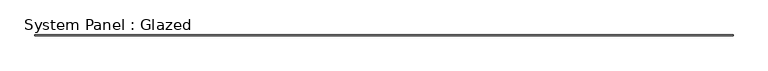
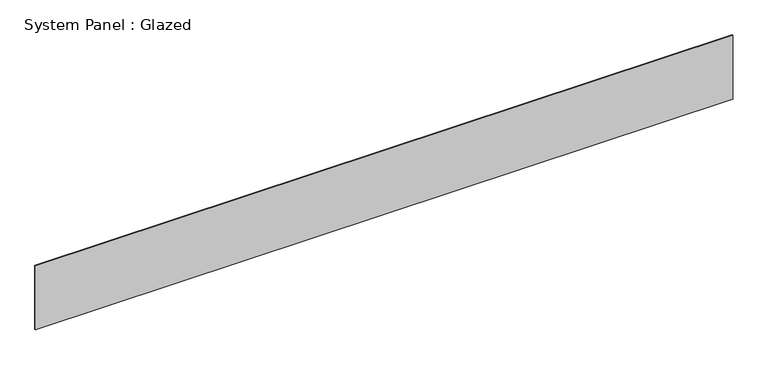
"""IFC4 building model written with IfcOpenShell, lengths in millimetres: plate geometry, System Panel : Glazed."""

from ifc_helpers import new_model, si_unit, origin, origin_with_axes, place, context, project, spatial, polyline, outline, extrude, source, transform, mapped, element, save


def system_panel_glazed_ba49168f(model_context):
    return source(origin(), model_context, "Body", "SweptSolid", [
        extrude(outline(polyline([(11049.0, 19.05), (-11049.0, 19.05), (-11049.0, 44.45), (11049.0, 44.45), (11049.0, 19.05)])), origin_with_axes(), (0.0, 0.0, 1.0), 2133.6),
    ])


if __name__ == "__main__":
    model = new_model("IFC4")
    model_context = context("Model", 3, world=origin())
    ifc_project = project(units=[si_unit("LENGTHUNIT", "METRE", prefix="MILLI")], contexts=[model_context])
    site = spatial("IfcSite", under=ifc_project)
    building = spatial("IfcBuilding", under=site)
    placement = place(None, origin())
    system_panel_glazed_shape = system_panel_glazed_ba49168f(model_context)
    element("IfcPlate", 1, ObjectType="System Panel : Glazed", at=placement, inside=building, context=model_context, shape_type="MappedRepresentation", body=[
        mapped(system_panel_glazed_shape, transform((0.0, 0.0, 0.0), x_axis=(1.0, 0.0, 0.0), y_axis=(0.0, 1.0, 0.0), z_axis=(0.0, 0.0, 1.0))),
    ])
    save(model, "model.ifc")

# Revit data of these elements
# Type "System Panel : Glazed"
#   Construction Type Id = "GSP4R"
#   Analytic Construction = "1/8 in Pilkington single glazing"
#   Visual Light Transmittance = 0.9
#   Solar Heat Gain Coefficient = 0.86
#   Heat Transfer Coefficient (U) = 1.18115 BTU/(h·ft²·°F)
# Element 1 (IfcPlate, "System Panel : Glazed")
#   Materials on its faces: "Glass"
# Materials
#   "Glass": class "Glass", colour RGB 0 128 192, transparency 0.75, Description = "Soda Lime Glass", Cost = 0
